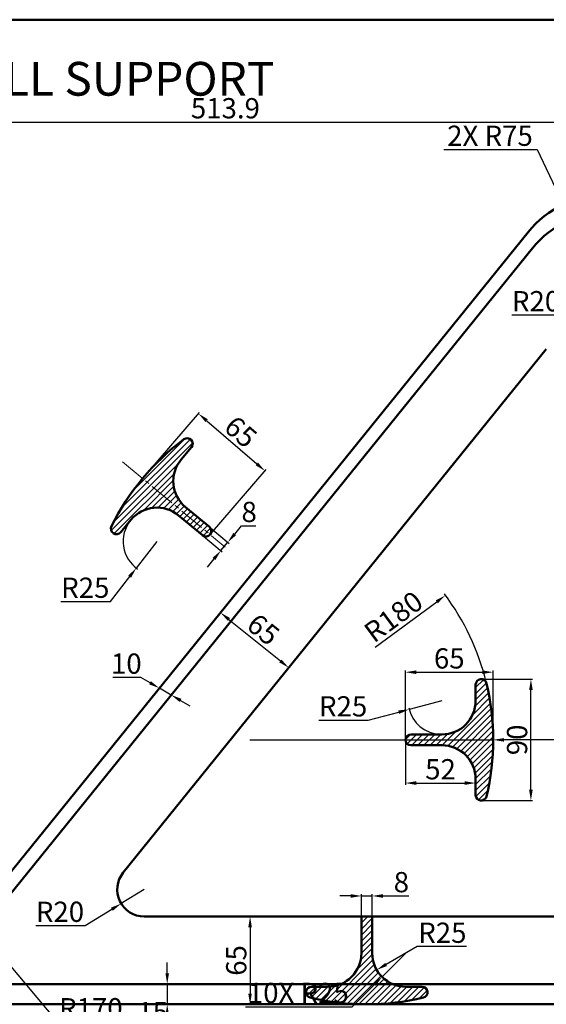
# Model space of a CAD drawing. Units: millimetres. Extents: x -60 to 1204, y -103 to 1006.
# Tile 3 of 4: x 452 to 842, y 277 to 1006. Entities that reach past the tile are written whole.
import ezdxf

# ---------------------------------------------------------------- set-up
doc = ezdxf.new("R2010")
doc.units = ezdxf.units.MM
doc.linetypes.add('CENTER2', pattern=[28.575, 19.05, -3.175, 3.175, -3.175])
for name, color, linetype, lineweight in [('M-CNTR', 1, 'CENTER2', 18), ('M-DIMS', 2, 'Continuous', 25), ('M-HATC', 8, 'Continuous', 18), ('M-OUTL', 7, 'Continuous', 50), ('M-TEXT', 7, 'Continuous', 25), ('M-TTLB', 7, 'Continuous', 50)]:
    doc.layers.add(name, color=color, linetype=linetype, lineweight=lineweight)
doc.styles.get("Standard").update_dxf_attribs({"font": 'arial.ttf'})
doc.dimstyles.new('ISO-25', dxfattribs={"dimtxt": 15, "dimasz": 8, "dimexe": 1.25, "dimexo": 0.625, "dimtad": 1, "dimtoh": 1, "dimdec": 0, "dimtxsty": 'Standard', "dimcen": 2.5, "dimadec": 0, "dimazin": 0, "dimtfac": 1, "dimtdec": 0, "dimtmove": 0, "dimatfit": 3, "dimfxl": 1, "dimarcsym": 0})

# ---------------------------------------------------------------- blocks, each defined once
blk = doc.blocks.new('*U4')
at = {"layer": 'M-CNTR', "color": 0, "transparency": 16777216}
blk.add_line((-32.4, 0), (154.61, 0), dxfattribs=at)
blk = doc.blocks.new('*D22')
at = {"layer": 'Defpoints', "color": 0, "transparency": 16777216}
for p in [(633.78, 671.83), (543.83, 667.06), (593.05, 624.6)]:
    blk.add_point(p, dxfattribs=at)
at = {"layer": 'M-DIMS', "color": 0, "lineweight": -2, "transparency": 16777216}
for p, q in [((544.23, 667.53), (585.37, 715.23)), ((590.61, 709.06), (627.72, 677.05)), ((593.46, 625.08), (634.6, 672.77))]:
    blk.add_line(p, q, dxfattribs=at)
at = {"layer": 'M-DIMS', "color": 0, "transparency": 16777216}
for points in [[(591.48, 710.07), (589.74, 708.05), (584.55, 714.28)], [(628.59, 678.06), (626.85, 676.04), (633.78, 671.83)]]:
    blk.add_solid(points, dxfattribs=at)
at = {"layer": 'M-DIMS', "color": 0, "transparency": 16777216, "insert": (614.58, 699.33), "char_height": 15, "attachment_point": 5, "rotation": 319.22559}
blk.add_mtext('65', dxfattribs=at)
blk = doc.blocks.new('*D23')
at = {"layer": 'Defpoints', "color": 0, "transparency": 16777216}
for p in [(802.67, 522.71), (737.67, 472.57), (802.67, 472.57)]:
    blk.add_point(p, dxfattribs=at)
at = {"layer": 'M-DIMS', "color": 0, "lineweight": -2, "transparency": 16777216}
for p, q in [((737.67, 473.19), (737.67, 523.96)), ((745.67, 522.71), (794.67, 522.71)), ((802.67, 473.19), (802.67, 523.96))]:
    blk.add_line(p, q, dxfattribs=at)
at = {"layer": 'M-DIMS', "color": 0, "transparency": 16777216}
for points in [[(745.67, 524.04), (745.67, 521.37), (737.67, 522.71)], [(794.67, 524.04), (794.67, 521.37), (802.67, 522.71)]]:
    blk.add_solid(points, dxfattribs=at)
at = {"layer": 'M-DIMS', "color": 0, "transparency": 16777216, "insert": (770.17, 530.99), "char_height": 15, "attachment_point": 5}
blk.add_mtext('65', dxfattribs=at)
blk = doc.blocks.new('*D24')
at = {"layer": 'Defpoints', "color": 0, "transparency": 16777216}
for p in [(793.28, 517.54), (830.58, 517.54), (793.76, 427.57)]:
    blk.add_point(p, dxfattribs=at)
at = {"layer": 'M-DIMS', "color": 0, "lineweight": -2, "transparency": 16777216}
for p, q in [((793.91, 517.54), (831.83, 517.54)), ((830.58, 435.57), (830.58, 509.54)), ((794.39, 427.57), (831.83, 427.57))]:
    blk.add_line(p, q, dxfattribs=at)
at = {"layer": 'M-DIMS', "color": 0, "transparency": 16777216}
for points in [[(829.25, 509.54), (831.92, 509.54), (830.58, 517.54)], [(829.25, 435.57), (831.92, 435.57), (830.58, 427.57)]]:
    blk.add_solid(points, dxfattribs=at)
at = {"layer": 'M-DIMS', "color": 0, "transparency": 16777216, "insert": (822.3, 472.56), "char_height": 15, "attachment_point": 5, "rotation": 90}
blk.add_mtext('90', dxfattribs=at)
blk = doc.blocks.new('*D25')
at = {"layer": 'Defpoints', "color": 0, "transparency": 16777216}
for p in [(737.71, 473.12), (789.67, 440.59), (789.67, 437.61)]:
    blk.add_point(p, dxfattribs=at)
at = {"layer": 'M-DIMS', "color": 0, "lineweight": -2, "transparency": 16777216}
for p, q in [((737.71, 472.5), (737.71, 439.34)), ((745.71, 440.59), (781.67, 440.59)), ((789.67, 438.24), (789.67, 441.84))]:
    blk.add_line(p, q, dxfattribs=at)
at = {"layer": 'M-DIMS', "color": 0, "transparency": 16777216}
for points in [[(745.71, 441.92), (745.71, 439.25), (737.71, 440.59)], [(781.67, 441.92), (781.67, 439.25), (789.67, 440.59)]]:
    blk.add_solid(points, dxfattribs=at)
at = {"layer": 'M-DIMS', "color": 0, "transparency": 16777216, "insert": (763.69, 448.87), "char_height": 15, "attachment_point": 5}
blk.add_mtext('52', dxfattribs=at)
blk = doc.blocks.new('*D26')
at = {"layer": 'Defpoints', "color": 0, "transparency": 16777216}
for p in [(767.35, 579.66), (622.67, 472.57)]:
    blk.add_point(p, dxfattribs=at)
at = {"layer": 'M-DIMS', "color": 0, "lineweight": -2, "transparency": 16777216}
blk.add_line((715.35, 541.17), (760.92, 574.9), dxfattribs=at)
blk.add_arc((622.67, 472.57), 180, 13.64736, 36.90707, dxfattribs=at)
at = {"layer": 'M-DIMS', "color": 0, "transparency": 16777216}
blk.add_solid([(760.13, 575.97), (761.71, 573.83), (767.35, 579.66)], dxfattribs=at)
at = {"layer": 'M-DIMS', "color": 0, "transparency": 16777216, "insert": (729.99, 562.31), "char_height": 15, "attachment_point": 5, "rotation": 36.50918}
blk.add_mtext('R180', dxfattribs=at)
blk = doc.blocks.new('*D27')
at = {"layer": 'Defpoints', "color": 0, "transparency": 16777216}
for p in [(764.67, 501.57), (740.5, 495.18)]:
    blk.add_point(p, dxfattribs=at)
at = {"layer": 'M-DIMS', "color": 0, "lineweight": -2, "transparency": 16777216}
for p, q in [((764.67, 501.57), (740.5, 495.18)), ((710.22, 487.18), (732.77, 493.14)), ((673.64, 487.18), (710.22, 487.18))]:
    blk.add_line(p, q, dxfattribs=at)
blk.add_arc((764.67, 501.57), 25, 191.93694, 268.56761, dxfattribs=at)
at = {"layer": 'M-DIMS', "color": 0, "transparency": 16777216}
blk.add_solid([(732.43, 494.43), (733.11, 491.85), (740.5, 495.18)], dxfattribs=at)
at = {"layer": 'M-DIMS', "color": 0, "transparency": 16777216, "insert": (691.62, 495.47), "char_height": 15, "attachment_point": 5}
blk.add_mtext('R25', dxfattribs=at)
blk = doc.blocks.new('*D28')
at = {"layer": 'Defpoints', "color": 0, "transparency": 16777216}
for p in [(583.75, 637.65), (578.63, 631.5), (606.23, 618.93)]:
    blk.add_point(p, dxfattribs=at)
at = {"layer": 'M-DIMS', "color": 0, "lineweight": -2, "transparency": 16777216}
for p, q in [((584.23, 637.25), (607.19, 618.13)), ((579.11, 631.1), (602.07, 611.98)), ((611.35, 625.08), (616.47, 631.23)), ((616.47, 631.23), (626.98, 631.23)), ((601.11, 612.78), (606.23, 618.93)), ((595.99, 606.63), (590.88, 600.48))]:
    blk.add_line(p, q, dxfattribs=at)
at = {"layer": 'M-DIMS', "color": 0, "transparency": 16777216}
for points in [[(610.32, 625.93), (612.37, 624.22), (606.23, 618.93)], [(594.97, 607.49), (597.02, 605.78), (601.11, 612.78)]]:
    blk.add_solid(points, dxfattribs=at)
at = {"layer": 'M-DIMS', "color": 0, "transparency": 16777216, "insert": (622.04, 639.51), "char_height": 15, "attachment_point": 5}
blk.add_mtext('8', dxfattribs=at)
blk = doc.blocks.new('*D29')
at = {"layer": 'Defpoints', "color": 0, "transparency": 16777216}
for p in [(553.79, 619.64), (538.51, 599.86)]:
    blk.add_point(p, dxfattribs=at)
at = {"layer": 'M-DIMS', "color": 0, "lineweight": -2, "transparency": 16777216}
for p, q in [((553.79, 619.64), (538.51, 599.86)), ((519.36, 575.08), (533.62, 593.53)), ((482.78, 575.08), (519.36, 575.08))]:
    blk.add_line(p, q, dxfattribs=at)
blk.add_arc((553.79, 619.64), 25, 141.65598, 235.16945, dxfattribs=at)
at = {"layer": 'M-DIMS', "color": 0, "transparency": 16777216}
blk.add_solid([(532.56, 594.35), (534.67, 592.72), (538.51, 599.86)], dxfattribs=at)
at = {"layer": 'M-DIMS', "color": 0, "transparency": 16777216, "insert": (500.76, 583.36), "char_height": 15, "attachment_point": 5}
blk.add_mtext('R25', dxfattribs=at)
blk = doc.blocks.new('*D30')
at = {"layer": 'Defpoints', "color": 0, "transparency": 16777216}
for p in [(600.83, 566.84), (651.4, 526), (651.4, 526)]:
    blk.add_point(p, dxfattribs=at)
at = {"layer": 'M-DIMS', "color": 0, "lineweight": -2, "transparency": 16777216}
for p, q in [((601.22, 567.32), (601.62, 567.81)), ((607.06, 561.81), (645.18, 531.03)), ((651.79, 526.49), (652.19, 526.97))]:
    blk.add_line(p, q, dxfattribs=at)
at = {"layer": 'M-DIMS', "color": 0, "transparency": 16777216}
for points in [[(607.89, 562.85), (606.22, 560.77), (600.83, 566.84)], [(646.01, 532.06), (644.34, 529.99), (651.4, 526)]]:
    blk.add_solid(points, dxfattribs=at)
at = {"layer": 'M-DIMS', "color": 0, "transparency": 16777216, "insert": (631.32, 552.86), "char_height": 15, "attachment_point": 5, "rotation": 321.07566}
blk.add_mtext('65', dxfattribs=at)
blk = doc.blocks.new('*D31')
at = {"layer": 'Defpoints', "color": 0, "transparency": 16777216}
for p in [(555.62, 510.86), (555.62, 510.86), (564.39, 505.8)]:
    blk.add_point(p, dxfattribs=at)
at = {"layer": 'M-DIMS', "color": 0, "lineweight": -2, "transparency": 16777216}
for p, q in [((541.77, 518.86), (521.12, 518.86)), ((548.69, 514.86), (541.77, 518.86)), ((564.39, 505.8), (555.62, 510.86)), ((555.93, 511.4), (556.25, 511.94)), ((564.7, 506.34), (565.01, 506.88)), ((571.32, 501.8), (578.24, 497.8))]:
    blk.add_line(p, q, dxfattribs=at)
at = {"layer": 'M-DIMS', "color": 0, "transparency": 16777216}
for points in [[(549.36, 516.01), (548.03, 513.7), (555.62, 510.86)], [(571.98, 502.95), (570.65, 500.64), (564.39, 505.8)]]:
    blk.add_solid(points, dxfattribs=at)
at = {"layer": 'M-DIMS', "color": 0, "transparency": 16777216, "insert": (531.13, 527.14), "char_height": 15, "attachment_point": 5}
blk.add_mtext('10', dxfattribs=at)
blk = doc.blocks.new('*D32')
at = {"layer": 'Defpoints', "color": 0, "transparency": 16777216}
for p in [(635.95, 341.66), (622.73, 276.66), (635.95, 276.66)]:
    blk.add_point(p, dxfattribs=at)
at = {"layer": 'M-DIMS', "color": 0, "lineweight": -2, "transparency": 16777216}
for p, q in [((635.32, 341.66), (621.48, 341.66)), ((622.73, 333.66), (622.73, 284.66)), ((635.32, 276.66), (621.48, 276.66))]:
    blk.add_line(p, q, dxfattribs=at)
at = {"layer": 'M-DIMS', "color": 0, "transparency": 16777216}
for points in [[(621.4, 333.66), (624.06, 333.66), (622.73, 341.66)], [(621.4, 284.66), (624.06, 284.66), (622.73, 276.66)]]:
    blk.add_solid(points, dxfattribs=at)
at = {"layer": 'M-DIMS', "color": 0, "transparency": 16777216, "insert": (614.45, 309.16), "char_height": 15, "attachment_point": 5, "rotation": 90}
blk.add_mtext('65', dxfattribs=at)
blk = doc.blocks.new('*D33')
at = {"layer": 'Defpoints', "color": 0, "transparency": 16777216}
for p in [(561.41, 291.66), (561.41, 276.66), (561.41, 276.66)]:
    blk.add_point(p, dxfattribs=at)
at = {"layer": 'M-DIMS', "color": 0, "lineweight": -2, "transparency": 16777216}
for p, q in [((561.41, 299.66), (561.41, 307.66)), ((561.41, 291.66), (561.41, 276.66)), ((562.03, 291.66), (562.66, 291.66)), ((562.03, 276.66), (562.66, 276.66)), ((561.41, 268.66), (561.41, 260.66)), ((561.41, 260.66), (540.6, 260.66))]:
    blk.add_line(p, q, dxfattribs=at)
at = {"layer": 'M-DIMS', "color": 0, "transparency": 16777216}
for points in [[(560.08, 299.66), (562.74, 299.66), (561.41, 291.66)], [(560.08, 268.66), (562.74, 268.66), (561.41, 276.66)]]:
    blk.add_solid(points, dxfattribs=at)
at = {"layer": 'M-DIMS', "color": 0, "transparency": 16777216, "insert": (550.69, 268.95), "char_height": 15, "attachment_point": 5}
blk.add_mtext('15', dxfattribs=at)
blk = doc.blocks.new('*D34')
at = {"layer": 'Defpoints', "color": 0, "transparency": 16777216}
for p in [(713.13, 356.93), (705.13, 341.66), (713.13, 341.66)]:
    blk.add_point(p, dxfattribs=at)
at = {"layer": 'M-DIMS', "color": 0, "lineweight": -2, "transparency": 16777216}
for p, q in [((705.13, 342.29), (705.13, 358.18)), ((713.13, 342.29), (713.13, 358.18)), ((697.13, 356.93), (689.13, 356.93)), ((705.13, 356.93), (713.13, 356.93)), ((721.13, 356.93), (740.26, 356.93))]:
    blk.add_line(p, q, dxfattribs=at)
at = {"layer": 'M-DIMS', "color": 0, "transparency": 16777216}
for points in [[(697.13, 358.27), (697.13, 355.6), (705.13, 356.93)], [(721.13, 358.27), (721.13, 355.6), (713.13, 356.93)]]:
    blk.add_solid(points, dxfattribs=at)
at = {"layer": 'M-DIMS', "color": 0, "transparency": 16777216, "insert": (734.69, 365.22), "char_height": 15, "attachment_point": 5}
blk.add_mtext('8', dxfattribs=at)
blk = doc.blocks.new('*D35')
at = {"layer": 'Defpoints', "color": 0, "transparency": 16777216}
for p in [(738.13, 314.66), (716.48, 302.16)]:
    blk.add_point(p, dxfattribs=at)
at = {"layer": 'M-DIMS', "color": 0, "lineweight": -2, "transparency": 16777216}
for p, q in [((746.44, 319.47), (723.4, 306.16)), ((783.02, 319.47), (746.44, 319.47))]:
    blk.add_line(p, q, dxfattribs=at)
at = {"layer": 'M-DIMS', "color": 0, "transparency": 16777216}
blk.add_solid([(722.74, 307.32), (724.07, 305.01), (716.48, 302.16)], dxfattribs=at)
at = {"layer": 'M-DIMS', "color": 0, "transparency": 16777216, "insert": (765.04, 327.75), "char_height": 15, "attachment_point": 5}
blk.add_mtext('R25', dxfattribs=at)
blk = doc.blocks.new('*D46')
at = {"layer": 'Defpoints', "color": 0, "transparency": 16777216}
for p in [(855.11, 769.26), (857.53, 749.41)]:
    blk.add_point(p, dxfattribs=at)
at = {"layer": 'M-DIMS', "color": 0, "lineweight": -2, "transparency": 16777216}
for p, q in [((816.49, 787.37), (852.9, 787.37)), ((852.9, 787.37), (854.14, 777.2)), ((857.53, 749.41), (855.11, 769.26))]:
    blk.add_line(p, q, dxfattribs=at)
at = {"layer": 'M-DIMS', "color": 0, "transparency": 16777216}
blk.add_solid([(855.47, 777.36), (852.82, 777.04), (855.11, 769.26)], dxfattribs=at)
at = {"layer": 'M-DIMS', "color": 0, "transparency": 16777216, "insert": (834.38, 795.65), "char_height": 15, "attachment_point": 5}
blk.add_mtext('R20', dxfattribs=at)
blk = doc.blocks.new('*D47')
at = {"layer": 'Defpoints', "color": 0, "transparency": 16777216}
for p in [(544.39, 361.66), (527.31, 351.27)]:
    blk.add_point(p, dxfattribs=at)
at = {"layer": 'M-DIMS', "color": 0, "lineweight": -2, "transparency": 16777216}
for p, q in [((544.39, 361.66), (527.31, 351.27)), ((500.56, 334.98), (520.47, 347.11)), ((464.14, 334.98), (500.56, 334.98))]:
    blk.add_line(p, q, dxfattribs=at)
at = {"layer": 'M-DIMS', "color": 0, "transparency": 16777216}
blk.add_solid([(519.78, 348.25), (521.17, 345.97), (527.31, 351.27)], dxfattribs=at)
at = {"layer": 'M-DIMS', "color": 0, "transparency": 16777216, "insert": (482.03, 343.27), "char_height": 15, "attachment_point": 5}
blk.add_mtext('R20', dxfattribs=at)
blk = doc.blocks.new('RIB-SECTION')
for p, q in [((52, 74), (52, 85.91)), ((4, 49), (27, 49)), ((4, 41), (27, 41)), ((52, 16), (52, 4.09))]:
    blk.add_line(p, q)
for centre, radius, start, end in [((56.09, 85.91), 4.09, 13.44842, 180), ((-115, 45), 180, 346.55158, 13.44842), ((27, 74), 25, 270, 0), ((4, 45), 4, 90, 270), ((27, 16), 25, 0, 90), ((56.09, 4.09), 4.09, 180, 346.55158)]:
    blk.add_arc(centre, radius, start, end)
blk = doc.blocks.new('*D68')
at = {"layer": 'Defpoints', "color": 0, "transparency": 16777216}
for p in [(861.39, 930.31), (861.39, 175.77), (347.53, 107.92)]:
    blk.add_point(p, dxfattribs=at)
at = {"layer": 'M-DIMS', "color": 0, "lineweight": -2, "transparency": 16777216}
for p, q in [((347.53, 108.55), (347.53, 931.56)), ((355.53, 930.31), (853.39, 930.31)), ((861.39, 176.39), (861.39, 931.56))]:
    blk.add_line(p, q, dxfattribs=at)
at = {"layer": 'M-DIMS', "color": 0, "transparency": 16777216}
for points in [[(355.53, 931.65), (355.53, 928.98), (347.53, 930.31)], [(853.39, 931.65), (853.39, 928.98), (861.39, 930.31)]]:
    blk.add_solid(points, dxfattribs=at)
at = {"layer": 'M-DIMS', "color": 0, "transparency": 16777216, "insert": (604.46, 938.6), "char_height": 15, "attachment_point": 5}
blk.add_mtext('513.9', dxfattribs=at)
blk = doc.blocks.new('*D70')
at = {"layer": 'Defpoints', "color": 0, "transparency": 16777216}
for p in [(622.67, 472.57), (802.67, 472.57)]:
    blk.add_point(p, dxfattribs=at)
at = {"layer": 'M-DIMS', "color": 0, "lineweight": -2, "transparency": 16777216}
for p, q in [((622.67, 472.57), (802.67, 472.57)), ((910.67, 472.57), (810.67, 472.57)), ((991.58, 472.57), (910.67, 472.57))]:
    blk.add_line(p, q, dxfattribs=at)
at = {"layer": 'M-DIMS', "color": 0, "transparency": 16777216}
blk.add_solid([(810.67, 473.9), (810.67, 471.24), (802.67, 472.57)], dxfattribs=at)
at = {"layer": 'M-DIMS', "color": 0, "transparency": 16777216, "insert": (951.44, 480.85), "char_height": 15, "attachment_point": 5}
blk.add_mtext('4X R180', dxfattribs=at)
blk = doc.blocks.new('*D71')
at = {"layer": 'Defpoints', "color": 0, "transparency": 16777216}
for p in [(305.45, 471.66), (414.89, 341.57)]:
    blk.add_point(p, dxfattribs=at)
at = {"layer": 'M-DIMS', "color": 0, "lineweight": -2, "transparency": 16777216}
for p, q in [((305.45, 471.66), (414.89, 341.57)), ((480.54, 263.51), (420.04, 335.45)), ((528.62, 263.51), (480.54, 263.51))]:
    blk.add_line(p, q, dxfattribs=at)
at = {"layer": 'M-DIMS', "color": 0, "transparency": 16777216}
blk.add_solid([(421.06, 336.31), (419.01, 334.59), (414.89, 341.57)], dxfattribs=at)
at = {"layer": 'M-DIMS', "color": 0, "transparency": 16777216, "insert": (504.89, 271.8), "char_height": 15, "attachment_point": 5}
blk.add_mtext('R170', dxfattribs=at)
blk = doc.blocks.new('*D72')
at = {"layer": 'Defpoints', "color": 0, "transparency": 16777216}
for p in [(854.55, 869.34), (886.88, 801.66)]:
    blk.add_point(p, dxfattribs=at)
at = {"layer": 'M-DIMS', "color": 0, "lineweight": -2, "transparency": 16777216}
for p, q in [((766.08, 909.94), (835.15, 909.94)), ((835.15, 909.94), (851.1, 876.56)), ((886.88, 801.66), (854.55, 869.34))]:
    blk.add_line(p, q, dxfattribs=at)
at = {"layer": 'M-DIMS', "color": 0, "transparency": 16777216}
blk.add_solid([(852.3, 877.13), (849.9, 875.98), (854.55, 869.34)], dxfattribs=at)
at = {"layer": 'M-DIMS', "color": 0, "transparency": 16777216, "insert": (800.3, 918.22), "char_height": 15, "attachment_point": 5}
blk.add_mtext('2X R75', dxfattribs=at)
blk = doc.blocks.new('*D75')
at = {"layer": 'Defpoints', "color": 0, "transparency": 16777216}
for p in [(738.13, 314.66), (720.45, 296.99)]:
    blk.add_point(p, dxfattribs=at)
at = {"layer": 'M-DIMS', "color": 0, "lineweight": -2, "transparency": 16777216}
for p, q in [((738.13, 314.66), (720.45, 296.99)), ((698.3, 274.84), (714.79, 291.33)), ((619.25, 274.84), (698.3, 274.84))]:
    blk.add_line(p, q, dxfattribs=at)
at = {"layer": 'M-DIMS', "color": 0, "transparency": 16777216}
blk.add_solid([(713.85, 292.27), (715.73, 290.39), (720.45, 296.99)], dxfattribs=at)
at = {"layer": 'M-DIMS', "color": 0, "transparency": 16777216, "insert": (658.46, 283.13), "char_height": 15, "attachment_point": 5}
blk.add_mtext('10X R25', dxfattribs=at)

msp = doc.modelspace()

# ---------------------------------------------------------------- hatches: boundary and pattern name
at = {"layer": 'M-HATC'}
h = msp.add_hatch(dxfattribs=at)
h.set_pattern_fill('ANSI31', color=256)
h.paths.add_polyline_path([(571.6885, 680.2142), (579.3095, 689.369, 0.889025), (573.72, 695.2592, 0.05874724), (543.1433, 666.2437), (593.0989, 624.6571, 0.41421356), (592.5839, 630.2904), (574.9073, 645.0057, -0.41421356)])
h.paths.add_polyline_path([(543.1433, 666.2437, 0.05874724), (520.1532, 630.9125, 0.889025), (526.9594, 626.4837), (534.5804, 635.6385, -0.41421356), (569.789, 638.8573), (587.4655, 624.1421, 0.41421356), (593.0989, 624.6571)])
h = msp.add_hatch(dxfattribs=at)
h.set_pattern_fill('ANSI31', color=256)
h.paths.add_polyline_path([(797.737, 514.4325, 0.889025), (789.6727, 513.4817), (789.6727, 501.5699, -0.41421356), (764.6727, 476.5699), (741.6727, 476.5699, 0.41421356), (737.6727, 472.5699), (802.6727, 472.5699, 0.05874724)])
h.paths.add_polyline_path([(802.6727, 472.5699), (737.6727, 472.5699, 0.41421356), (741.6727, 468.5699), (764.6727, 468.5699, -0.41421356), (789.6727, 443.5699), (789.6727, 431.6582, 0.889025), (797.737, 430.7074, 0.05874724)])
h = msp.add_hatch(dxfattribs=at)
h.set_pattern_fill('ANSI31', color=256)
h.paths.add_polyline_path([(728.3278, 291.6642), (689.9238, 291.6642, -0.10102051), (680.1258, 289.6642), (668.214, 289.6642, 0.889025), (667.2632, 281.5998, 0.11790138), (750.9884, 281.5998, 0.889025), (750.0376, 289.6642), (738.1258, 289.6642, -0.10102051)])
h.paths.add_polyline_path([(713.1258, 314.6642), (713.1258, 341.6642), (705.1258, 341.6642), (705.1258, 314.6642, -0.30061413), (689.9238, 291.6642), (728.3278, 291.6642, -0.30061413)])

# ---------------------------------------------------------------- linework, layer by layer
at = {"layer": 'M-CNTR'}
msp.add_line((528.1969, 678.6861), (604.2853, 615.3447), dxfattribs=at)
at = {"layer": 'M-OUTL', "ltscale": 0.5}
for p, q in [((437.7092, 364.8543), (828.5326, 848.7862)), ((404.6048, 307.9471), (831.6952, 836.7862)), ((528.8312, 374.2301), (841.9712, 761.9716))]:
    msp.add_line(p, q, dxfattribs=at)
at = {"layer": 'M-OUTL'}
for p, q in [((544.3907, 341.6642), (857.5307, 341.6642)), ((705.1258, 341.6642), (705.1258, 314.6642)), ((713.1258, 341.6642), (713.1258, 314.6642)), ((292.5307, 291.6642), (1002.5307, 291.6642)), ((680.1258, 289.6642), (668.214, 289.6642)), ((738.1258, 289.6642), (750.0376, 289.6642)), ((292.5307, 276.6642), (1002.5307, 276.6642))]:
    msp.add_line(p, q, dxfattribs=at)
at = {"layer": 'M-OUTL', "ltscale": 0.5}
for centre in [(886.8808, 801.6642), (890.0435, 789.6642)]:
    msp.add_arc(centre, 75, 90, 141.0756607, dxfattribs=at)
at = {"layer": 'M-OUTL'}
for centre, radius, start, end in [((544.3907, 361.6642), 20, 141.0756607, 270), ((680.1258, 314.6642), 25, 270, 0), ((738.1258, 314.6642), 25, 180, 270), ((668.214, 285.576), 4.0882, 90, 256.5515825), ((750.0376, 285.576), 4.0882, 283.4484175, 90), ((709.1258, 456.6642), 180, 256.5515825, 283.4484175)]:
    msp.add_arc(centre, radius, start, end, dxfattribs=at)
at = {"layer": 'M-TTLB'}
msp.add_lwpolyline([(-59.5454, 1006.1383), (1204.2342, 1006.1383), (1204.2342, -103.2116), (-59.5454, -103.2116)], close=True, dxfattribs=at)

# ---------------------------------------------------------------- block references
at = {"layer": 'M-CNTR'}
msp.add_blockref('*U4', (753.1727, 472.5699), dxfattribs=at)
at = {"layer": 'M-OUTL', "rotation": 140.223582112875}
msp.add_blockref('RIB-SECTION', (621.8887, 659.2411), dxfattribs=at)
at = {"layer": 'M-OUTL'}
msp.add_blockref('RIB-SECTION', (737.673, 427.571), dxfattribs=at)

# ---------------------------------------------------------------- texts
at = {"layer": 'M-TEXT', "insert": (389.9254, 974.8573), "char_height": 25, "attachment_point": 1}
msp.add_mtext_dynamic_manual_height_columns('WALL SUPPORT', width=382.720281, gutter_width=12.5, heights=[0], dxfattribs=at)

# ---------------------------------------------------------------- dimensions: what is measured, and where the dimension line sits
at = {"layer": 'M-DIMS'}
for base, p1, p2, override, picture, middle in [((861.3892, 930.3142), (347.5307, 107.9202), (861.3892, 175.7691), {"dimdec": 1, "dimlfac": 1, "dimrnd": 0, "dimzin": 0, "dimdsep": 46, "dimlunit": 2}, '*D68', (604.46, 938.6029)), ((802.6727, 522.7056), (737.6727, 472.5699), (802.6727, 472.5699), {"dimclrd": 0, "dimclre": 0, "dimclrt": 0}, '*D23', (770.1727, 530.9892)), ((789.6727, 440.5861), (737.7114, 473.125), (789.6727, 437.6141), {"dimclrd": 0, "dimclre": 0, "dimclrt": 0}, '*D25', (763.692, 448.8697)), ((713.1258, 356.9332), (705.1258, 341.6642), (713.1258, 341.6642), {"dimclrd": 0, "dimclre": 0, "dimclrt": 0}, '*D34', (734.6928, 365.2168))]:
    dim = msp.add_linear_dim(base=base, p1=p1, p2=p2, dimstyle='ISO-25', override=override, dxfattribs=at)
    dim.commit()
    dim.dimension.update_dxf_attribs({"geometry": picture, "text_midpoint": middle})
for center, mpoint, text, picture, middle in [((886.8808, 801.6642), (854.5481, 869.3369), '2X <>', '*D72', (800.3027, 909.9405)), ((622.6727, 472.5699), (802.6727, 472.57), '4X <>', '*D70', (910.6727, 472.57))]:
    dim = msp.add_radius_dim(center=center, mpoint=mpoint, text=text, dimstyle='ISO-25', override={"dimdec": 0, "dimlfac": 1, "dimrnd": 0, "dimzin": 0, "dimdsep": 46, "dimlunit": 2}, dxfattribs=at)
    dim.commit()
    dim.dimension.update_dxf_attribs({"geometry": picture, "text_midpoint": middle, "dimtype": 164})
for center, mpoint, override, picture, middle in [((857.5307, 749.4057), (855.1116, 769.2589), {"dimclrd": 0, "dimclre": 0, "dimclrt": 0}, '*D46', (834.3841, 787.3695)), ((622.6727, 472.5699), (767.3497, 579.6612), {"dimclrd": 0, "dimclre": 0, "dimclrt": 0}, '*D26', (734.9198, 555.6563)), ((305.4532, 471.6642), (414.8855, 341.5697), {"dimdec": 0, "dimlfac": 1, "dimrnd": 0, "dimzin": 0, "dimdsep": 46, "dimlunit": 2}, '*D71', (504.8926, 263.513)), ((738.1258, 314.6642), (716.4752, 302.1642), {"dimclrd": 0, "dimclre": 0, "dimclrt": 0}, '*D35', (765.0443, 319.4654))]:
    dim = msp.add_radius_dim(center=center, mpoint=mpoint, dimstyle='ISO-25', override=override, dxfattribs=at)
    dim.commit()
    dim.dimension.update_dxf_attribs({"geometry": picture, "text_midpoint": middle, "dimtype": 164})
for p1, p2, distance, picture, middle in [((543.8256, 667.0583), (593.0539, 624.6039), 62.3594, '*D22', (614.5754, 699.3281)), ((578.6272, 631.4997), (583.7456, 637.6481), -29.2574, '*D28', (622.035, 639.5097)), ((600.8316, 566.8384), (651.4001, 525.9994), 0, '*D30', (631.3204, 552.8633)), ((564.3882, 505.7968), (555.6218, 510.858), 0, '*D31', (531.1285, 527.1416)), ((635.9494, 341.6642), (635.9494, 276.6642), -13.2186, '*D32', (614.4472, 309.1642)), ((561.4091, 291.6642), (561.4091, 276.6642), 0, '*D33', (550.6903, 268.9478))]:
    dim = msp.add_aligned_dim(p1=p1, p2=p2, distance=distance, dimstyle='ISO-25', override={"dimclrd": 0, "dimclre": 0, "dimclrt": 0}, dxfattribs=at)
    dim.commit()
    dim.dimension.update_dxf_attribs({"geometry": picture, "text_midpoint": middle})
for center, mpoint, picture, middle in [((553.7941, 619.6436), (538.5076, 599.8618), '*D29', (500.7558, 583.365)), ((764.6727, 501.5699), (740.5023, 495.1831), '*D27', (691.6218, 495.4659)), ((544.3907, 361.6642), (527.3065, 351.2656), '*D47', (482.0345, 343.2665))]:
    dim = msp.add_radius_dim(center=center, mpoint=mpoint, dimstyle='ISO-25', override={"dimclrd": 0, "dimclre": 0, "dimclrt": 0}, dxfattribs=at)
    dim.commit()
    dim.dimension.update_dxf_attribs({"geometry": picture, "text_midpoint": middle})
dim = msp.add_linear_dim(base=(830.5835, 517.5418), p1=(793.7609, 427.5699), p2=(793.2822, 517.5418), angle=90, dimstyle='ISO-25', override={"dimclrd": 0, "dimclre": 0, "dimclrt": 0}, dxfattribs=at)
dim.commit()
dim.dimension.update_dxf_attribs({"geometry": '*D24', "text_midpoint": (822.2999, 472.5559)})
dim = msp.add_radius_dim(center=(738.1258, 314.6642), mpoint=(720.4478, 296.9868), text='10X <>', dimstyle='ISO-25', override={"dimdec": 0, "dimlfac": 1, "dimrnd": 0, "dimzin": 0, "dimdsep": 46, "dimlunit": 2}, dxfattribs=at)
dim.commit()
dim.dimension.update_dxf_attribs({"geometry": '*D75', "text_midpoint": (658.464, 283.1262)})

doc.saveas('drawing.dxf')
